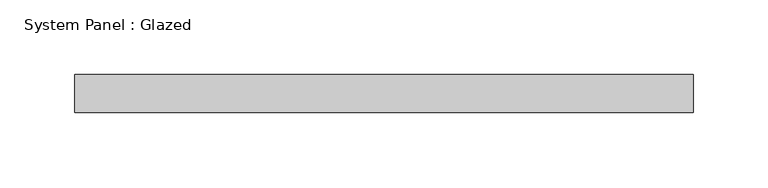
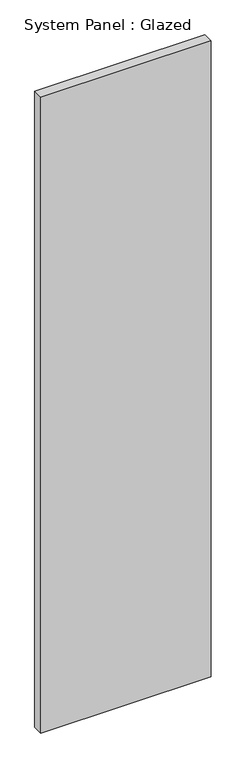
"""IFC4 building model written with IfcOpenShell, lengths in millimetres: plate geometry, System Panel : Glazed."""

from ifc_helpers import new_model, si_unit, origin, origin_with_axes, place, context, project, spatial, polyline, outline, extrude, source, transform, mapped, element, save


def system_panel_glazed_ae4f7e76(model_context):
    return source(origin(), model_context, "Body", "SweptSolid", [
        extrude(outline(polyline([(206.375, 19.05), (-206.375, 19.05), (-206.375, 44.45), (206.375, 44.45), (206.375, 19.05)])), origin_with_axes(), (0.0, 0.0, 1.0), 1630.2747989),
    ])


if __name__ == "__main__":
    model = new_model("IFC4")
    model_context = context("Model", 3, world=origin())
    ifc_project = project(units=[si_unit("LENGTHUNIT", "METRE", prefix="MILLI")], contexts=[model_context])
    site = spatial("IfcSite", under=ifc_project)
    building = spatial("IfcBuilding", under=site)
    placement = place(None, origin())
    system_panel_glazed_shape = system_panel_glazed_ae4f7e76(model_context)
    element("IfcPlate", 1, ObjectType="System Panel : Glazed", at=placement, inside=building, context=model_context, shape_type="MappedRepresentation", body=[
        mapped(system_panel_glazed_shape, transform((0.0, 0.0, 0.0), x_axis=(1.0, 0.0, 0.0), y_axis=(0.0, 1.0, 0.0), z_axis=(0.0, 0.0, 1.0))),
    ])
    save(model, "model.ifc")

# Revit data of these elements
# Type "System Panel : Glazed"
#   Construction Type Id = "GSP4R"
#   Analytic Construction = "1/8 in Pilkington single glazing"
#   Visual Light Transmittance = 0.9
#   Solar Heat Gain Coefficient = 0.86
#   Heat Transfer Coefficient (U) = 1.18115 BTU/(h·ft²·°F)
#   Define Thermal Properties by = 1
# Element 1 (IfcPlate, "System Panel : Glazed")
#   Materials on its faces: "Glass"
# Materials
#   "Glass": class "Glass", colour RGB 0 128 192, transparency 0.75, Description = "Soda Lime Glass", Cost = 0
